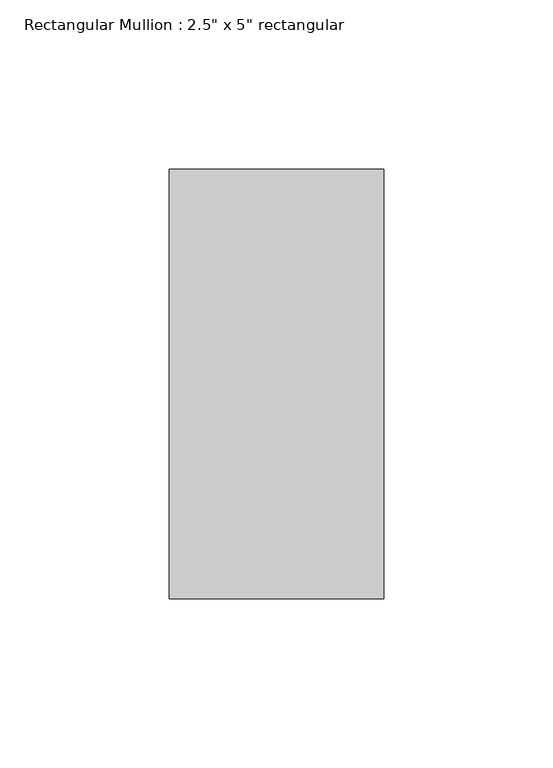
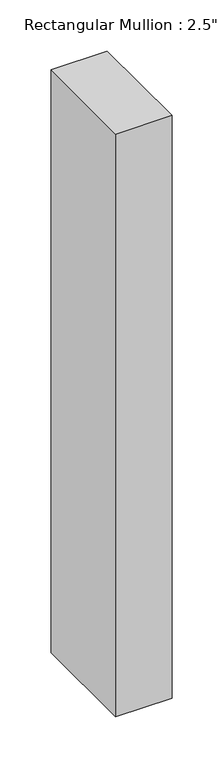
"""IFC4 building model written with IfcOpenShell, lengths in millimetres: member geometry."""

from ifc_helpers import new_model, si_unit, frame, origin, place, context, project, spatial, polyline, outline, extrude, source, transform, mapped, element, save


def member_d4cc7fbf(model_context):
    return source(origin(), model_context, "Body", "SweptSolid", [
        extrude(outline(polyline([(0.0, 63.5), (0.0, -63.5), (-63.5, -63.5), (-63.5, 63.5), (0.0, 63.5)])), frame((0.0, 0.0, -696.9443895), z_axis=(0.0, 0.0, 1.0), x_axis=(1.0, 0.0, 0.0)), (0.0, 0.0, 1.0), 696.9443895),
    ])


if __name__ == "__main__":
    model = new_model("IFC4")
    model_context = context("Model", 3, world=origin())
    ifc_project = project(units=[si_unit("LENGTHUNIT", "METRE", prefix="MILLI")], contexts=[model_context])
    site = spatial("IfcSite", under=ifc_project)
    building = spatial("IfcBuilding", under=site)
    placement = place(None, origin())
    member_shape = member_d4cc7fbf(model_context)
    element("IfcMember", 1, ObjectType="Rectangular Mullion : 2.5\" x 5\" rectangular", at=placement, inside=building, context=model_context, shape_type="MappedRepresentation", body=[
        mapped(member_shape, transform((0.0, 0.0, 0.0), x_axis=(1.0, 0.0, 0.0), y_axis=(0.0, 1.0, 0.0), z_axis=(0.0, 0.0, 1.0))),
    ])
    save(model, "model.ifc")

# Revit data of these elements
# Type "Rectangular Mullion : 2.5\" x 5\" rectangular"
#   built-in parameter 1007304 = 0.416667 (stored number, unit not read)
#   built-in parameter 1007301 = 0.104167 (stored number, unit not read)
#   built-in parameter 1007300 = 0.104167 (stored number, unit not read)
# Element 1 (IfcMember, "Rectangular Mullion : 2.5\" x 5\" rectangular")
#   Materials on its faces: "Aluminum"
# Materials
#   "Aluminum": class "Metal", colour RGB 247 247 247, transparency 0, Description = "Aluminum 6061", Cost = 0
